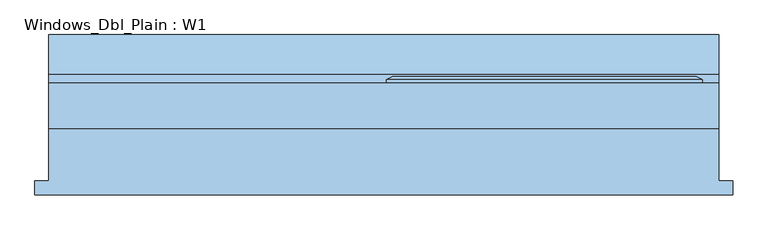
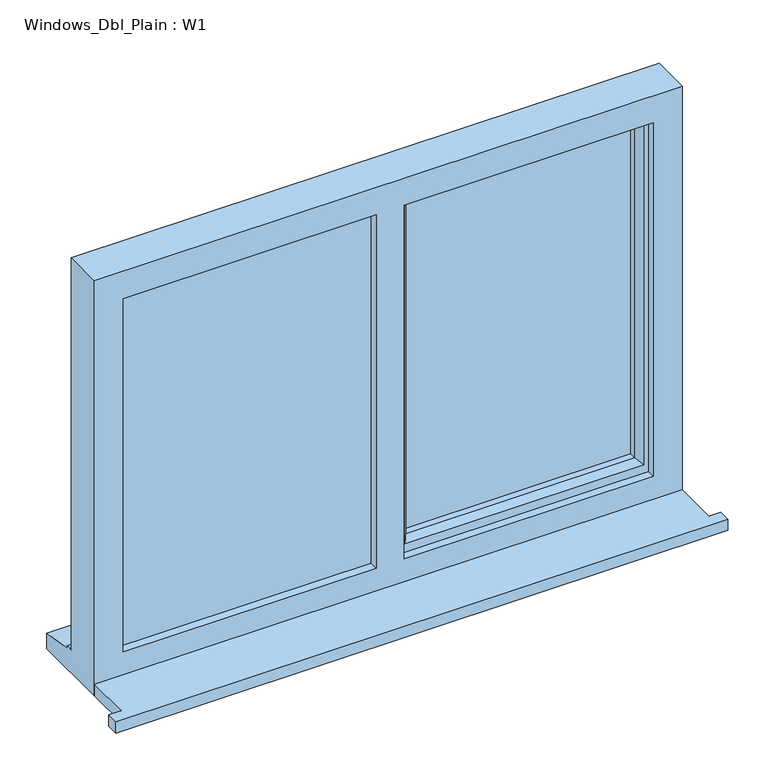
"""IFC4 building model written with IfcOpenShell, lengths in millimetres: window geometry, Windows_Dbl_Plain : W1."""

from ifc_helpers import new_model, si_unit, frame, origin, place, context, project, spatial, polyline, outline, extrude, faceted_brep, source, transform, mapped, element, save


def windows_dbl_plain_w1_9e0d93ab(model_context):
    return source(origin(), model_context, "Body", "SolidModel", [
        extrude(outline(polyline([(-919.6, -130.8434322), (-919.6, -105.8434322), (-894.6, -105.8434322), (-894.6, -10.2434322), (324.6, -10.2434322), (324.6, -105.8434322), (349.6, -105.8434322), (349.6, -130.8434322), (-919.6, -130.8434322)])), frame((0.0, 0.0, 1200.0), z_axis=(0.0, 0.0, 1.0), x_axis=(1.0, 0.0, 0.0)), (0.0, 0.0, 1.0), 25.0),
        faceted_brep([(-280.0, 72.7565678, 2080.0), (-280.0, 78.5300705, 2080.0), (-280.0, 78.5300705, 1253.0), (-280.0, 72.7565678, 1253.0), (-270.0, 7.7565678, 2070.0), (-270.0, 72.7565678, 2070.0), (-270.0, 72.7565678, 1263.0), (-270.0, 7.7565678, 1263.0), (-230.0, 22.2494677, 2030.0), (-240.1480377, 7.7565678, 2040.1480377), (-240.1480377, 7.7565678, 1292.8519623), (-230.0, 22.2494677, 1303.0), (-230.0, 36.7565678, 2030.0), (-230.0, 36.7565678, 1303.0), (-240.0, 60.7565678, 2040.0), (-240.0, 36.7565678, 2040.0), (-240.0, 36.7565678, 1293.0), (-240.0, 60.7565678, 1293.0), (-230.0, 78.5300705, 2030.0), (-230.0, 60.7565678, 2030.0), (-230.0, 60.7565678, 1303.0), (-230.0, 78.5300705, 1303.0), (-247.4457548, 84.3035732, 2047.4457548), (-247.4457548, 84.3035732, 1285.5542452), (-269.2153903, 84.3035732, 2069.2153903), (-269.2153903, 84.3035732, 1263.7846097), (294.6, 78.5300705, 1253.0), (294.6, 72.7565678, 1253.0), (284.6, 72.7565678, 1263.0), (284.6, 7.7565678, 1263.0), (254.7480377, 7.7565678, 1292.8519623), (244.6, 22.2494677, 1303.0), (244.6, 36.7565678, 1303.0), (254.6, 36.7565678, 1293.0), (254.6, 60.7565678, 1293.0), (244.6, 60.7565678, 1303.0), (244.6, 78.5300705, 1303.0), (262.0457548, 84.3035732, 1285.5542452), (283.8153903, 84.3035732, 1263.7846097), (294.6, 78.5300705, 2080.0), (294.6, 72.7565678, 2080.0), (284.6, 72.7565678, 2070.0), (284.6, 7.7565678, 2070.0), (254.7480377, 7.7565678, 2040.1480377), (244.6, 22.2494677, 2030.0), (244.6, 36.7565678, 2030.0), (254.6, 36.7565678, 2040.0), (254.6, 60.7565678, 2040.0), (244.6, 60.7565678, 2030.0), (244.6, 78.5300705, 2030.0), (262.0457548, 84.3035732, 2047.4457548), (283.8153903, 84.3035732, 2069.2153903)], [[[0, 1, 2, 3]], [[4, 5, 6, 7]], [[8, 9, 10, 11]], [[12, 8, 11, 13]], [[14, 15, 16, 17]], [[18, 19, 20, 21]], [[22, 18, 21, 23]], [[1, 24, 25, 2]], [[3, 2, 26, 27]], [[7, 6, 28, 29]], [[11, 10, 30, 31]], [[13, 11, 31, 32]], [[17, 16, 33, 34]], [[21, 20, 35, 36]], [[23, 21, 36, 37]], [[2, 25, 38, 26]], [[27, 26, 39, 40]], [[29, 28, 41, 42]], [[31, 30, 43, 44]], [[32, 31, 44, 45]], [[34, 33, 46, 47]], [[36, 35, 48, 49]], [[37, 36, 49, 50]], [[26, 38, 51, 39]], [[40, 39, 1, 0]], [[3, 27, 40, 0], [5, 41, 28, 6]], [[42, 41, 5, 4]], [[7, 29, 42, 4], [9, 43, 30, 10]], [[44, 43, 9, 8]], [[45, 44, 8, 12]], [[15, 46, 33, 16], [13, 32, 45, 12]], [[47, 46, 15, 14]], [[17, 34, 47, 14], [19, 48, 35, 20]], [[49, 48, 19, 18]], [[50, 49, 18, 22]], [[24, 51, 38, 25], [23, 37, 50, 22]], [[39, 51, 24, 1]]]),
        extrude(outline(polyline([(2050.0, -310.0), (2070.0, -310.0), (2070.0, -854.6), (1263.0, -854.6), (1263.0, -310.0), (1283.0, -310.0), (1283.0, -834.6), (2050.0, -834.6), (2050.0, -310.0)])), frame((0.0, 31.7565678, 0.0), z_axis=(0.0, 1.0, 0.0), x_axis=(0.0, 0.0, 1.0)), (0.0, 0.0, 1.0), 41.0),
        faceted_brep([(324.6, -10.2434322, 2110.0), (-894.6, -10.2434322, 2110.0), (-894.6, -10.2434322, 1200.0), (324.6, -10.2434322, 1200.0), (264.6, -10.2434322, 2050.0), (264.6, -10.2434322, 1275.0), (-252.0, -10.2434322, 1275.0), (-252.0, -10.2434322, 2050.0), (-310.0, -10.2434322, 2050.0), (-310.0, -10.2434322, 1275.0), (-834.6, -10.2434322, 1275.0), (-834.6, -10.2434322, 2050.0), (-894.6, 72.7565678, 2110.0), (-894.6, 72.7565678, 1251.0), (-894.6, 87.7565678, 1249.68767), (-894.6, 87.7565678, 1244.7449676), (-894.6, 160.2565678, 1233.8088847), (-894.6, 160.2565678, 1200.0), (324.6, 72.7565678, 2110.0), (324.6, 72.7565678, 1251.0), (-854.6, 72.7565678, 2070.0), (-854.6, 72.7565678, 1263.0), (-310.0, 72.7565678, 1263.0), (-310.0, 72.7565678, 2070.0), (-270.0, 72.7565678, 2070.0), (-270.0, 72.7565678, 1263.0), (284.6, 72.7565678, 1263.0), (284.6, 72.7565678, 2070.0), (-854.6, 7.7565678, 2070.0), (-854.6, 7.7565678, 1263.0), (-300.0, 7.7565678, 2070.0), (-300.0, 7.7565678, 1263.0), (-310.0, 7.7565678, 2050.0), (-834.6, 7.7565678, 2050.0), (-834.6, 7.7565678, 1275.0), (-310.0, 7.7565678, 1275.0), (-270.0, 7.7565678, 2070.0), (284.6, 7.7565678, 2070.0), (284.6, 7.7565678, 1263.0), (-270.0, 7.7565678, 1263.0), (264.6, 7.7565678, 2050.0), (-252.0, 7.7565678, 2050.0), (-252.0, 7.7565678, 1275.0), (264.6, 7.7565678, 1275.0), (-310.0, 31.7565678, 2070.0), (-300.0, 31.7565678, 2070.0), (324.6, 160.2565678, 1200.0), (324.6, 160.2565678, 1233.8088847), (324.6, 87.7565678, 1244.7449676), (324.6, 87.7565678, 1249.68767), (-300.0, 31.7565678, 1263.0), (-310.0, 31.7565678, 1263.0)], [[[0, 1, 2, 3], [4, 5, 6, 7], [8, 9, 10, 11]], [[2, 1, 12, 13, 14, 15, 16, 17]], [[13, 12, 18, 19], [20, 21, 22, 23], [24, 25, 26, 27]], [[21, 20, 28, 29]], [[28, 30, 31, 29], [32, 33, 34, 35]], [[36, 37, 38, 39], [40, 41, 42, 43]], [[33, 11, 10, 34]], [[1, 0, 18, 12]], [[28, 20, 23, 44, 45, 30]], [[27, 37, 36, 24]], [[11, 33, 32, 8]], [[40, 4, 7, 41]], [[19, 18, 0, 3, 46, 47, 48, 49]], [[27, 26, 38, 37]], [[4, 40, 43, 5]], [[45, 50, 31, 30]], [[50, 45, 44, 51]], [[51, 44, 23, 22]], [[25, 24, 36, 39]], [[41, 7, 6, 42]], [[8, 32, 35, 9]], [[46, 3, 2, 17]], [[47, 46, 17, 16]], [[48, 47, 16, 15]], [[49, 48, 15, 14]], [[19, 49, 14, 13]], [[22, 21, 29, 31, 50, 51]], [[26, 25, 39, 38]], [[6, 5, 43, 42]], [[35, 34, 10, 9]]]),
        extrude(outline(polyline([(-854.6, 31.7565678), (-300.0, 31.7565678), (-300.0, 7.7565678), (-854.6, 7.7565678), (-854.6, 31.7565678)])), frame((0.0, 0.0, 1263.0), z_axis=(0.0, 0.0, 1.0), x_axis=(1.0, 0.0, 0.0)), (0.0, 0.0, 1.0), 807.0),
        extrude(outline(polyline([(254.6, 36.7565678), (-240.0, 36.7565678), (-240.0, 60.7565678), (254.6, 60.7565678), (254.6, 36.7565678)])), frame((0.0, 0.0, 1293.0), z_axis=(0.0, 0.0, 1.0), x_axis=(1.0, 0.0, 0.0)), (0.0, 0.0, 1.0), 747.0),
    ])


if __name__ == "__main__":
    model = new_model("IFC4")
    model_context = context("Model", 3, world=origin())
    ifc_project = project(units=[si_unit("LENGTHUNIT", "METRE", prefix="MILLI")], contexts=[model_context])
    site = spatial("IfcSite", under=ifc_project)
    building = spatial("IfcBuilding", under=site)
    placement = place(None, origin())
    windows_dbl_plain_w1_shape = windows_dbl_plain_w1_9e0d93ab(model_context)
    element("IfcWindow", 1, ObjectType="Windows_Dbl_Plain : W1", at=placement, inside=building, context=model_context, shape_type="MappedRepresentation", body=[
        mapped(windows_dbl_plain_w1_shape, transform((0.0, 0.0, 0.0), x_axis=(1.0, 0.0, 0.0), y_axis=(0.0, 1.0, 0.0), z_axis=(0.0, 0.0, 1.0))),
    ])
    save(model, "model.ifc")

# Revit data of these elements
# Type "Windows_Dbl_Plain : W1"
#   Type Mark = "56"
#   Operation = "DoublePanelVertical"
#   Construction Type Id = "GSP4R"
#   Manufacturer = "Revit"
#   Keynote = "L10"
#   Analytic Construction = "1/8 in Pilkington single glazing"
#   Wrap Layers (Ext) from Ext = 0.336286 ft
#   Wrap Layers (Int) from Ext = 0.582349 ft
#   Window Board Projection = 0.082021 ft
#   Window Board Extension = 0.082021 ft
#   Visual Light Transmittance = 0.9
#   Solar Heat Gain Coefficient = 0.78
#   Rough Width = 4.0 ft
#   Rough Height = 2.985564 ft
#   Height = 2.985564 ft
#   Width = 4.0 ft
#   Heat Transfer Coefficient (U) = 3.6886 W/(m²·K)
#   Glazing Thickness = 0.07874 ft
#   FrameOffset - External = 0.164042 ft
#   Frame Depth = 0.213255 ft
#   Default Head Height = 6.922572 ft
#   Cill Depth = 0.287073 ft
#   Cavity Closer Width = 0.164042 ft
#   Cavity Closer Offset from Ext = 0.336286 ft
#   Cavity Closer Depth = 0.278871 ft
#   Vis - Cavity Closers = yes
#   Define Thermal Properties by = 1
#   Material Trim = Window Frame
#   Material Glass = Glass
#   Material Frame = Window Frame
#   Wall Closure = (empty or 0)
# Element 1 (IfcWindow, "Windows_Dbl_Plain : W1")
#   Materials on its faces: "Window Frame", "Glass"
# Materials
#   "Window Frame": colour RGB 249 249 249, transparency 0, Keynote = "L10", Cost = 0
#   "Glass": class "Glass", colour RGB 0 128 192, transparency 0.9, Description = "Soda Lime Glass", Cost = 0
